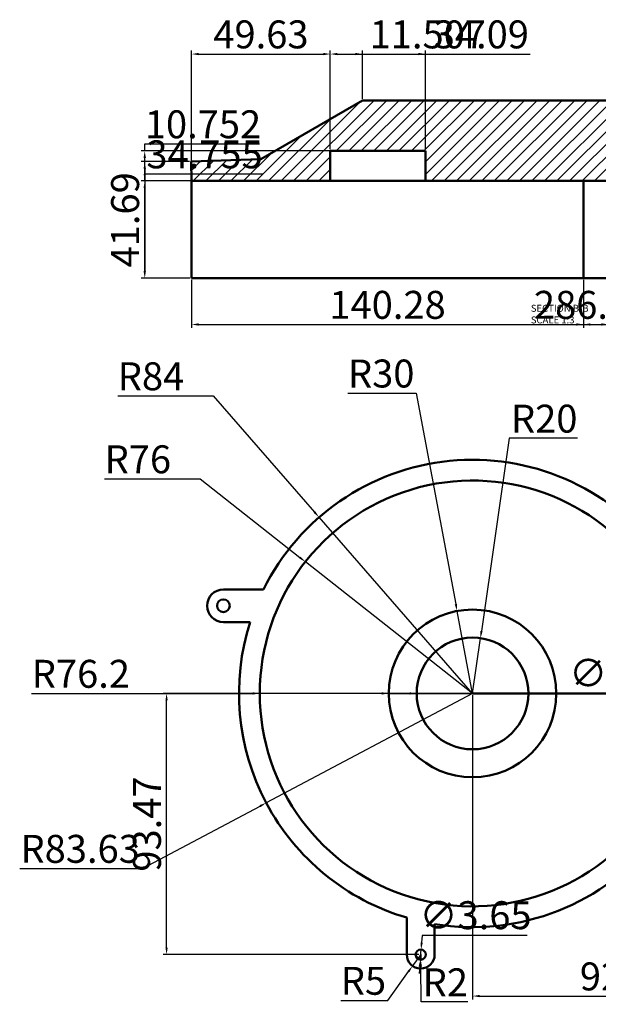
# Model space of a CAD drawing. Units: millimetres. Extents: x 828 to 2987, y 979 to 1807.
# Tile 1 of 6: x 851 to 1058, y 1108 to 1460. Entities that reach past the tile are written whole.
import ezdxf

# ---------------------------------------------------------------- set-up
doc = ezdxf.new("R2010")
doc.units = ezdxf.units.MM
for name, color, linetype, lineweight in [('M-DIMS', 2, 'Continuous', 25), ('M-HATC', 8, 'Continuous', 18), ('M-OUTL', 7, 'Continuous', 50), ('M-TEXT', 3, 'Continuous', 25)]:
    doc.layers.add(name, color=color, linetype=linetype, lineweight=lineweight)
doc.styles.get("Standard").update_dxf_attribs({"font": 'arial.ttf'})
doc.dimstyles.new('ISO-25', dxfattribs={"dimtxt": 10, "dimasz": 2.5, "dimexe": 1.25, "dimexo": 0.625, "dimtad": 1, "dimtoh": 1, "dimdec": 0, "dimtxsty": 'Standard', "dimcen": 2.5, "dimadec": 0, "dimazin": 0, "dimtfac": 1, "dimtdec": 0, "dimtmove": 0, "dimatfit": 3, "dimfxl": 1, "dimarcsym": 0})

# ---------------------------------------------------------------- blocks, each defined once
blk = doc.blocks.new('*D17')
at = {"layer": 'Defpoints', "color": 0, "transparency": 16777216}
for p in [(1013.21, 1219.26), (1105.21, 1219.26), (1105.21, 1110.96)]:
    blk.add_point(p, dxfattribs=at)
at = {"layer": 'M-DIMS', "color": 0, "lineweight": -2, "transparency": 16777216}
for p, q in [((1013.21, 1218.63), (1013.21, 1109.71)), ((1105.21, 1218.63), (1105.21, 1109.71)), ((1015.71, 1110.96), (1102.71, 1110.96))]:
    blk.add_line(p, q, dxfattribs=at)
at = {"layer": 'M-DIMS', "color": 0, "transparency": 16777216}
for points in [[(1015.71, 1111.37), (1015.71, 1110.54), (1013.21, 1110.96)], [(1102.71, 1111.37), (1102.71, 1110.54), (1105.21, 1110.96)]]:
    blk.add_solid(points, dxfattribs=at)
at = {"layer": 'M-DIMS', "color": 0, "transparency": 16777216, "insert": (1059.21, 1116.69), "char_height": 10, "attachment_point": 5}
blk.add_mtext('92', dxfattribs=at)
blk = doc.blocks.new('*D18')
at = {"layer": 'Defpoints', "color": 0, "transparency": 16777216}
for p in [(958.25, 1282.29), (1013.21, 1219.26)]:
    blk.add_point(p, dxfattribs=at)
at = {"layer": 'M-DIMS', "color": 0, "lineweight": -2, "transparency": 16777216}
for p, q in [((886.14, 1325.74), (920.35, 1325.74)), ((920.35, 1325.74), (956.61, 1284.17)), ((1013.21, 1219.26), (958.25, 1282.29))]:
    blk.add_line(p, q, dxfattribs=at)
at = {"layer": 'M-DIMS', "color": 0, "transparency": 16777216}
blk.add_solid([(956.92, 1284.44), (956.29, 1283.9), (958.25, 1282.29)], dxfattribs=at)
at = {"layer": 'M-DIMS', "color": 0, "transparency": 16777216, "insert": (898.07, 1331.47), "char_height": 10, "attachment_point": 5}
blk.add_mtext('R84', dxfattribs=at)
blk = doc.blocks.new('*D19')
at = {"layer": 'Defpoints', "color": 0, "transparency": 16777216}
for p in [(953.34, 1266.38), (1013.21, 1219.26)]:
    blk.add_point(p, dxfattribs=at)
at = {"layer": 'M-DIMS', "color": 0, "lineweight": -2, "transparency": 16777216}
for p, q in [((881.42, 1296.03), (915.66, 1296.03)), ((915.66, 1296.03), (951.37, 1267.92)), ((1013.21, 1219.26), (953.34, 1266.38))]:
    blk.add_line(p, q, dxfattribs=at)
at = {"layer": 'M-DIMS', "color": 0, "transparency": 16777216}
blk.add_solid([(951.63, 1268.25), (951.11, 1267.59), (953.34, 1266.38)], dxfattribs=at)
at = {"layer": 'M-DIMS', "color": 0, "transparency": 16777216, "insert": (893.36, 1301.76), "char_height": 10, "attachment_point": 5}
blk.add_mtext('R76', dxfattribs=at)
blk = doc.blocks.new('*D25')
at = {"layer": 'Defpoints', "color": 0, "transparency": 16777216}
for p in [(994.65, 1125.79), (991.73, 1121.73)]:
    blk.add_point(p, dxfattribs=at)
at = {"layer": 'M-DIMS', "color": 0, "lineweight": -2, "transparency": 16777216}
for p, q in [((994.65, 1125.79), (991.73, 1121.73)), ((982.88, 1109.41), (990.27, 1119.7)), ((966.05, 1109.41), (982.88, 1109.41))]:
    blk.add_line(p, q, dxfattribs=at)
at = {"layer": 'M-DIMS', "color": 0, "transparency": 16777216}
blk.add_solid([(989.93, 1119.94), (990.61, 1119.45), (991.73, 1121.73)], dxfattribs=at)
at = {"layer": 'M-DIMS', "color": 0, "transparency": 16777216, "insert": (974.15, 1115.12), "char_height": 10, "attachment_point": 5}
blk.add_mtext('R5', dxfattribs=at)
blk = doc.blocks.new('*D26')
at = {"layer": 'Defpoints', "color": 0, "transparency": 16777216}
for p in [(994.65, 1125.79), (994.67, 1123.96)]:
    blk.add_point(p, dxfattribs=at)
at = {"layer": 'M-DIMS', "color": 0, "lineweight": -2, "transparency": 16777216}
for p, q in [((994.65, 1125.79), (994.67, 1123.96)), ((994.83, 1108.92), (994.69, 1121.46)), ((1011.47, 1108.92), (994.83, 1108.92))]:
    blk.add_line(p, q, dxfattribs=at)
at = {"layer": 'M-DIMS', "color": 0, "transparency": 16777216}
blk.add_solid([(995.11, 1121.47), (994.28, 1121.46), (994.67, 1123.96)], dxfattribs=at)
at = {"layer": 'M-DIMS', "color": 0, "transparency": 16777216, "insert": (1003.46, 1114.57), "char_height": 10, "attachment_point": 5}
blk.add_mtext('R2', dxfattribs=at)
blk = doc.blocks.new('*D27')
at = {"layer": 'Defpoints', "color": 0, "transparency": 16777216}
for p in [(1007.69, 1248.75), (1013.21, 1219.26)]:
    blk.add_point(p, dxfattribs=at)
at = {"layer": 'M-DIMS', "color": 0, "lineweight": -2, "transparency": 16777216}
for p, q in [((968.58, 1326.71), (993.07, 1326.71)), ((993.07, 1326.71), (1007.23, 1251.2)), ((1013.21, 1219.26), (1007.69, 1248.75))]:
    blk.add_line(p, q, dxfattribs=at)
at = {"layer": 'M-DIMS', "color": 0, "transparency": 16777216}
blk.add_solid([(1007.64, 1251.28), (1006.82, 1251.13), (1007.69, 1248.75)], dxfattribs=at)
at = {"layer": 'M-DIMS', "color": 0, "transparency": 16777216, "insert": (980.51, 1332.45), "char_height": 10, "attachment_point": 5}
blk.add_mtext('R30', dxfattribs=at)
blk = doc.blocks.new('*D28')
at = {"layer": 'Defpoints', "color": 0, "transparency": 16777216}
for p in [(1016.06, 1239.06), (1013.21, 1219.26)]:
    blk.add_point(p, dxfattribs=at)
at = {"layer": 'M-DIMS', "color": 0, "lineweight": -2, "transparency": 16777216}
for p, q in [((1026.32, 1310.58), (1016.41, 1241.53)), ((1050.81, 1310.58), (1026.32, 1310.58)), ((1013.21, 1219.26), (1016.06, 1239.06))]:
    blk.add_line(p, q, dxfattribs=at)
at = {"layer": 'M-DIMS', "color": 0, "transparency": 16777216}
blk.add_solid([(1016, 1241.59), (1016.82, 1241.47), (1016.06, 1239.06)], dxfattribs=at)
at = {"layer": 'M-DIMS', "color": 0, "transparency": 16777216, "insert": (1038.88, 1316.31), "char_height": 10, "attachment_point": 5}
blk.add_mtext('R20', dxfattribs=at)
blk = doc.blocks.new('*D77')
at = {"layer": 'Defpoints', "color": 0, "transparency": 16777216}
for p in [(903.65, 1219.26), (1013.21, 1219.26), (994.65, 1125.79)]:
    blk.add_point(p, dxfattribs=at)
at = {"layer": 'M-DIMS', "color": 0, "lineweight": -2, "transparency": 16777216}
for p, q in [((1012.59, 1219.26), (902.4, 1219.26)), ((903.65, 1128.29), (903.65, 1216.76)), ((994.02, 1125.79), (902.4, 1125.79))]:
    blk.add_line(p, q, dxfattribs=at)
at = {"layer": 'M-DIMS', "color": 0, "transparency": 16777216}
for points in [[(903.24, 1216.76), (904.07, 1216.76), (903.65, 1219.26)], [(903.24, 1128.29), (904.07, 1128.29), (903.65, 1125.79)]]:
    blk.add_solid(points, dxfattribs=at)
at = {"layer": 'M-DIMS', "color": 0, "transparency": 16777216, "insert": (897.92, 1172.52), "char_height": 10, "attachment_point": 5, "rotation": 90}
blk.add_mtext('93.47', dxfattribs=at)
blk = doc.blocks.new('*D80')
at = {"layer": 'Defpoints', "color": 0, "transparency": 16777216}
for p in [(912.63, 1367.9), (1199.4, 1367.9), (1199.4, 1351.3)]:
    blk.add_point(p, dxfattribs=at)
at = {"layer": 'M-DIMS', "color": 0, "lineweight": -2, "transparency": 16777216}
for p, q in [((912.63, 1367.28), (912.63, 1350.05)), ((1199.4, 1367.28), (1199.4, 1350.05)), ((915.13, 1351.3), (1196.9, 1351.3))]:
    blk.add_line(p, q, dxfattribs=at)
at = {"layer": 'M-DIMS', "color": 0, "transparency": 16777216}
for points in [[(915.13, 1351.72), (915.13, 1350.88), (912.63, 1351.3)], [(1196.9, 1351.72), (1196.9, 1350.88), (1199.4, 1351.3)]]:
    blk.add_solid(points, dxfattribs=at)
at = {"layer": 'M-DIMS', "color": 0, "transparency": 16777216, "insert": (1056.02, 1357.03), "char_height": 10, "attachment_point": 5}
blk.add_mtext('286.76', dxfattribs=at)
blk = doc.blocks.new('*D82')
at = {"layer": 'Defpoints', "color": 0, "transparency": 16777216}
for p in [(895.83, 1402.66), (912.63, 1402.66), (912.63, 1367.9)]:
    blk.add_point(p, dxfattribs=at)
at = {"layer": 'M-DIMS', "color": 0, "lineweight": -2, "transparency": 16777216}
for p, q in [((912.01, 1402.66), (894.58, 1402.66)), ((895.83, 1402.66), (895.83, 1405.16)), ((895.83, 1405.16), (938.04, 1405.16)), ((895.83, 1370.4), (895.83, 1400.16)), ((912.01, 1367.9), (894.58, 1367.9))]:
    blk.add_line(p, q, dxfattribs=at)
at = {"layer": 'M-DIMS', "color": 0, "transparency": 16777216}
for points in [[(895.42, 1400.16), (896.25, 1400.16), (895.83, 1402.66)], [(895.42, 1370.4), (896.25, 1370.4), (895.83, 1367.9)]]:
    blk.add_solid(points, dxfattribs=at)
at = {"layer": 'M-DIMS', "color": 0, "transparency": 16777216, "insert": (917.25, 1410.89), "char_height": 10, "attachment_point": 5}
blk.add_mtext('34.755', dxfattribs=at)
blk = doc.blocks.new('*D83')
at = {"layer": 'Defpoints', "color": 0, "transparency": 16777216}
for p in [(912.43, 1409.59), (895.83, 1367.9), (912.63, 1367.9)]:
    blk.add_point(p, dxfattribs=at)
at = {"layer": 'M-DIMS', "color": 0, "lineweight": -2, "transparency": 16777216}
for p, q in [((911.81, 1409.59), (894.58, 1409.59)), ((895.83, 1407.09), (895.83, 1370.4)), ((912.01, 1367.9), (894.58, 1367.9))]:
    blk.add_line(p, q, dxfattribs=at)
at = {"layer": 'M-DIMS', "color": 0, "transparency": 16777216}
for points in [[(895.42, 1407.09), (896.25, 1407.09), (895.83, 1409.59)], [(895.42, 1370.4), (896.25, 1370.4), (895.83, 1367.9)]]:
    blk.add_solid(points, dxfattribs=at)
at = {"layer": 'M-DIMS', "color": 0, "transparency": 16777216, "insert": (890.1, 1388.75), "char_height": 10, "attachment_point": 5, "rotation": 90}
blk.add_mtext('41.69', dxfattribs=at)
blk = doc.blocks.new('*D84')
at = {"layer": 'Defpoints', "color": 0, "transparency": 16777216}
for p in [(973.77, 1448.08), (973.77, 1431.48), (962.27, 1413.41)]:
    blk.add_point(p, dxfattribs=at)
at = {"layer": 'M-DIMS', "color": 0, "lineweight": -2, "transparency": 16777216}
for p, q in [((962.27, 1414.03), (962.27, 1449.33)), ((973.77, 1432.11), (973.77, 1449.33)), ((964.77, 1448.08), (971.27, 1448.08)), ((973.77, 1448.08), (1018.1, 1448.08))]:
    blk.add_line(p, q, dxfattribs=at)
at = {"layer": 'M-DIMS', "color": 0, "transparency": 16777216}
for points in [[(964.77, 1448.5), (964.77, 1447.67), (962.27, 1448.08)], [(971.27, 1448.5), (971.27, 1447.67), (973.77, 1448.08)]]:
    blk.add_solid(points, dxfattribs=at)
at = {"layer": 'M-DIMS', "color": 0, "transparency": 16777216, "insert": (997.19, 1453.81), "char_height": 10, "attachment_point": 5}
blk.add_mtext('11.507', dxfattribs=at)
blk = doc.blocks.new('*D85')
at = {"layer": 'Defpoints', "color": 0, "transparency": 16777216}
for p in [(962.27, 1448.08), (962.27, 1413.41), (912.63, 1402.66)]:
    blk.add_point(p, dxfattribs=at)
at = {"layer": 'M-DIMS', "color": 0, "lineweight": -2, "transparency": 16777216}
for p, q in [((912.63, 1403.28), (912.63, 1449.33)), ((962.27, 1414.03), (962.27, 1449.33)), ((915.13, 1448.08), (959.77, 1448.08))]:
    blk.add_line(p, q, dxfattribs=at)
at = {"layer": 'M-DIMS', "color": 0, "transparency": 16777216}
for points in [[(915.13, 1448.5), (915.13, 1447.67), (912.63, 1448.08)], [(959.77, 1448.5), (959.77, 1447.67), (962.27, 1448.08)]]:
    blk.add_solid(points, dxfattribs=at)
at = {"layer": 'M-DIMS', "color": 0, "transparency": 16777216, "insert": (937.45, 1453.82), "char_height": 10, "attachment_point": 5}
blk.add_mtext('49.63', dxfattribs=at)
blk = doc.blocks.new('*D86')
at = {"layer": 'Defpoints', "color": 0, "transparency": 16777216}
for p in [(996.36, 1448.08), (962.27, 1413.41), (996.36, 1413.41)]:
    blk.add_point(p, dxfattribs=at)
at = {"layer": 'M-DIMS', "color": 0, "lineweight": -2, "transparency": 16777216}
for p, q in [((962.27, 1414.03), (962.27, 1449.33)), ((996.36, 1414.03), (996.36, 1449.33)), ((964.77, 1448.08), (993.86, 1448.08)), ((996.36, 1448.08), (1033.87, 1448.08))]:
    blk.add_line(p, q, dxfattribs=at)
at = {"layer": 'M-DIMS', "color": 0, "transparency": 16777216}
for points in [[(964.77, 1448.5), (964.77, 1447.67), (962.27, 1448.08)], [(993.86, 1448.5), (993.86, 1447.67), (996.36, 1448.08)]]:
    blk.add_solid(points, dxfattribs=at)
at = {"layer": 'M-DIMS', "color": 0, "transparency": 16777216, "insert": (1016.36, 1453.82), "char_height": 10, "attachment_point": 5}
blk.add_mtext('34.09', dxfattribs=at)
blk = doc.blocks.new('*D87')
at = {"layer": 'Defpoints', "color": 0, "transparency": 16777216}
for p in [(895.83, 1413.41), (996.36, 1413.41), (996.36, 1402.66)]:
    blk.add_point(p, dxfattribs=at)
at = {"layer": 'M-DIMS', "color": 0, "lineweight": -2, "transparency": 16777216}
for p, q in [((995.73, 1413.41), (894.58, 1413.41)), ((895.83, 1413.41), (895.83, 1415.91)), ((895.83, 1415.91), (936.93, 1415.91)), ((895.83, 1405.16), (895.83, 1410.91)), ((995.73, 1402.66), (894.58, 1402.66))]:
    blk.add_line(p, q, dxfattribs=at)
at = {"layer": 'M-DIMS', "color": 0, "transparency": 16777216}
for points in [[(895.42, 1410.91), (896.25, 1410.91), (895.83, 1413.41)], [(895.42, 1405.16), (896.25, 1405.16), (895.83, 1402.66)]]:
    blk.add_solid(points, dxfattribs=at)
at = {"layer": 'M-DIMS', "color": 0, "transparency": 16777216, "insert": (916.69, 1421.64), "char_height": 10, "attachment_point": 5}
blk.add_mtext('10.752', dxfattribs=at)
blk = doc.blocks.new('*D91')
at = {"layer": 'Defpoints', "color": 0, "transparency": 16777216}
for p in [(912.63, 1367.9), (1052.92, 1367.9), (1052.92, 1351.3)]:
    blk.add_point(p, dxfattribs=at)
at = {"layer": 'M-DIMS', "color": 0, "lineweight": -2, "transparency": 16777216}
for p, q in [((912.63, 1367.28), (912.63, 1350.05)), ((1052.92, 1367.28), (1052.92, 1350.05)), ((915.13, 1351.3), (1050.42, 1351.3))]:
    blk.add_line(p, q, dxfattribs=at)
at = {"layer": 'M-DIMS', "color": 0, "transparency": 16777216}
for points in [[(915.13, 1351.72), (915.13, 1350.88), (912.63, 1351.3)], [(1050.42, 1351.72), (1050.42, 1350.88), (1052.92, 1351.3)]]:
    blk.add_solid(points, dxfattribs=at)
at = {"layer": 'M-DIMS', "color": 0, "transparency": 16777216, "insert": (982.78, 1357.03), "char_height": 10, "attachment_point": 5}
blk.add_mtext('140.28', dxfattribs=at)
blk = doc.blocks.new('*D92')
at = {"layer": 'Defpoints', "color": 0, "transparency": 16777216}
for p in [(1052.92, 1367.9), (1061.89, 1367.9), (1061.89, 1351.3)]:
    blk.add_point(p, dxfattribs=at)
at = {"layer": 'M-DIMS', "color": 0, "lineweight": -2, "transparency": 16777216}
for p, q in [((1052.92, 1367.28), (1052.92, 1350.05)), ((1061.89, 1367.28), (1061.89, 1350.05)), ((1055.42, 1351.3), (1059.39, 1351.3)), ((1061.89, 1351.3), (1091.63, 1351.3))]:
    blk.add_line(p, q, dxfattribs=at)
at = {"layer": 'M-DIMS', "color": 0, "transparency": 16777216}
for points in [[(1055.42, 1351.72), (1055.42, 1350.88), (1052.92, 1351.3)], [(1059.39, 1351.72), (1059.39, 1350.88), (1061.89, 1351.3)]]:
    blk.add_solid(points, dxfattribs=at)
at = {"layer": 'M-DIMS', "color": 0, "transparency": 16777216, "insert": (1078.01, 1357.03), "char_height": 10, "attachment_point": 5}
blk.add_mtext('8.97', dxfattribs=at)
blk = doc.blocks.new('*D124')
at = {"layer": 'Defpoints', "color": 0, "transparency": 16777216}
for p in [(1013.21, 1219.26), (939.32, 1180.1)]:
    blk.add_point(p, dxfattribs=at)
at = {"layer": 'M-DIMS', "color": 0, "lineweight": -2, "transparency": 16777216}
for p, q in [((1013.21, 1219.26), (939.32, 1180.1)), ((894.99, 1156.6), (937.12, 1178.93)), ((851.05, 1156.6), (894.99, 1156.6))]:
    blk.add_line(p, q, dxfattribs=at)
at = {"layer": 'M-DIMS', "color": 0, "transparency": 16777216}
blk.add_solid([(936.92, 1179.3), (937.31, 1178.56), (939.32, 1180.1)], dxfattribs=at)
at = {"layer": 'M-DIMS', "color": 0, "transparency": 16777216, "insert": (872.71, 1162.34), "char_height": 10, "attachment_point": 5}
blk.add_mtext('R83.63', dxfattribs=at)
blk = doc.blocks.new('*D125')
at = {"layer": 'Defpoints', "color": 0, "transparency": 16777216}
for p in [(937.02, 1219.26), (1013.21, 1219.26)]:
    blk.add_point(p, dxfattribs=at)
at = {"layer": 'M-DIMS', "color": 0, "lineweight": -2, "transparency": 16777216}
for p, q in [((855.24, 1219.26), (891.31, 1219.26)), ((891.31, 1219.26), (934.52, 1219.26)), ((1013.21, 1219.26), (937.02, 1219.26))]:
    blk.add_line(p, q, dxfattribs=at)
at = {"layer": 'M-DIMS', "color": 0, "transparency": 16777216}
blk.add_solid([(934.52, 1219.68), (934.52, 1218.84), (937.02, 1219.26)], dxfattribs=at)
at = {"layer": 'M-DIMS', "color": 0, "transparency": 16777216, "insert": (872.96, 1224.99), "char_height": 10, "attachment_point": 5}
blk.add_mtext('R76.2', dxfattribs=at)
blk = doc.blocks.new('*D126')
at = {"layer": 'Defpoints', "color": 0, "transparency": 16777216}
for p in [(983.21, 1219.26), (1043.21, 1219.26)]:
    blk.add_point(p, dxfattribs=at)
at = {"layer": 'M-DIMS', "color": 0, "lineweight": -2, "transparency": 16777216}
for p, q in [((980.71, 1219.26), (978.21, 1219.26)), ((983.21, 1219.26), (1043.21, 1219.26)), ((1061.21, 1219.26), (1045.71, 1219.26)), ((1087.01, 1219.26), (1061.21, 1219.26))]:
    blk.add_line(p, q, dxfattribs=at)
at = {"layer": 'M-DIMS', "color": 0, "transparency": 16777216}
for points in [[(980.71, 1219.68), (980.71, 1218.84), (983.21, 1219.26)], [(1045.71, 1219.68), (1045.71, 1218.84), (1043.21, 1219.26)]]:
    blk.add_solid(points, dxfattribs=at)
at = {"layer": 'M-DIMS', "color": 0, "transparency": 16777216, "insert": (1074.43, 1225.27), "char_height": 10, "attachment_point": 5}
blk.add_mtext('∅60', dxfattribs=at)
blk = doc.blocks.new('*D127')
at = {"layer": 'Defpoints', "color": 0, "transparency": 16777216}
for p in [(993.21, 1219.26), (1033.21, 1219.26)]:
    blk.add_point(p, dxfattribs=at)
at = {"layer": 'M-DIMS', "color": 0, "lineweight": -2, "transparency": 16777216}
for p, q in [((990.71, 1219.26), (988.21, 1219.26)), ((993.21, 1219.26), (1033.21, 1219.26)), ((1048.99, 1219.26), (1035.71, 1219.26)), ((1074.78, 1219.26), (1048.99, 1219.26))]:
    blk.add_line(p, q, dxfattribs=at)
at = {"layer": 'M-DIMS', "color": 0, "transparency": 16777216}
for points in [[(990.71, 1219.68), (990.71, 1218.84), (993.21, 1219.26)], [(1035.71, 1219.68), (1035.71, 1218.84), (1033.21, 1219.26)]]:
    blk.add_solid(points, dxfattribs=at)
at = {"layer": 'M-DIMS', "color": 0, "transparency": 16777216, "insert": (1062.2, 1225.27), "char_height": 10, "attachment_point": 5}
blk.add_mtext('∅40', dxfattribs=at)
blk = doc.blocks.new('*D132')
at = {"layer": 'Defpoints', "color": 0, "transparency": 16777216}
for p in [(994.79, 1127.61), (994.51, 1123.97)]:
    blk.add_point(p, dxfattribs=at)
at = {"layer": 'M-DIMS', "color": 0, "lineweight": -2, "transparency": 16777216}
for p, q in [((995.19, 1132.59), (994.99, 1130.1)), ((1032.74, 1132.59), (995.19, 1132.59)), ((994.51, 1123.97), (994.79, 1127.61)), ((994.31, 1121.48), (994.11, 1118.98))]:
    blk.add_line(p, q, dxfattribs=at)
at = {"layer": 'M-DIMS', "color": 0, "transparency": 16777216}
for points in [[(994.57, 1130.13), (995.4, 1130.07), (994.79, 1127.61)], [(993.89, 1121.51), (994.72, 1121.44), (994.51, 1123.97)]]:
    blk.add_solid(points, dxfattribs=at)
at = {"layer": 'M-DIMS', "color": 0, "transparency": 16777216, "insert": (1014.28, 1138.6), "char_height": 10, "attachment_point": 5}
blk.add_mtext('∅3.65', dxfattribs=at)

msp = doc.modelspace()

# ---------------------------------------------------------------- hatches: boundary and pattern name
at = {"layer": 'M-HATC'}
h = msp.add_hatch(dxfattribs=at)
h.set_pattern_fill('ANSI31', color=256)
h.paths.add_polyline_path([(962.2684, 1413.4084), (996.3583, 1413.4084), (996.3583, 1402.6561), (1084.8819, 1402.6561), (1084.8819, 1414.7818), (1117.3222, 1414.7818), (1117.3222, 1402.6561), (1194.3976, 1402.6561), (1194.3976, 1367.9009), (1199.3976, 1367.9009), (1199.3976, 1423.4818, -0.41421356), (1191.3976, 1431.4818), (1171.0768, 1431.4818), (1161.8287, 1415.4895, -0.59566696), (1156.5548, 1415.6369), (1148.5383, 1431.4818), (973.775, 1431.4818), (937.4085, 1410.469), (912.4339, 1409.5934), (912.6342, 1402.6561), (962.2684, 1402.6561)])

# ---------------------------------------------------------------- linework, layer by layer
at = {"layer": 'M-OUTL'}
for p, q in [((973.775, 1431.4818), (937.4085, 1410.469)), ((1191.3976, 1431.4818), (973.775, 1431.4818)), ((962.2684, 1402.6561), (962.2684, 1413.4084)), ((962.2684, 1413.4084), (996.3583, 1413.4084)), ((996.3583, 1413.4084), (996.3583, 1402.6561)), ((937.4085, 1410.469), (912.4339, 1409.5934)), ((912.4339, 1409.5934), (912.6342, 1402.6561)), ((1194.3976, 1402.6561), (912.6342, 1402.6561)), ((912.6342, 1367.9009), (912.6342, 1402.6561)), ((1052.9164, 1367.9009), (1052.9164, 1402.6561)), ((912.6342, 1367.9009), (1194.3976, 1367.9009)), ((923.9922, 1256.4847), (938.3309, 1256.4847)), ((923.9922, 1244.804), (933.5857, 1244.804)), ((1013.2149, 1219.2594), (1105.2149, 1219.2594)), ((989.6492, 1125.7871), (989.6492, 1139.0223)), ((999.6492, 1125.7871), (999.6492, 1136.7409))]:
    msp.add_line(p, q, dxfattribs=at)
for centre, radius in [((923.9922, 1250.6444), 2.2667), ((1013.2149, 1219.2594), 30), ((1013.2149, 1219.2594), 20), ((994.6492, 1125.7871), 1.8253)]:
    msp.add_circle(centre, radius, dxfattribs=at)
for centre, radius, start, end in [((1013.2149, 1219.2594), 83.6262, 37.706236, 153.567782), ((1013.2149, 1219.2594), 76.1927, 33.749512, 326.250488), ((923.9922, 1250.6444), 5.8403, 90, 270), ((1013.2149, 1219.2594), 83.6262, 162.214047, 253.632492), ((1013.2149, 1219.2594), 83.6262, 260.664363, 322.293764), ((994.6492, 1125.7871), 5, 180, 0)]:
    msp.add_arc(centre, radius, start, end, dxfattribs=at)

# ---------------------------------------------------------------- texts
at = {"layer": 'M-TEXT', "insert": (1034.0859, 1358.3458), "char_height": 2.5, "attachment_point": 1}
msp.add_mtext_dynamic_manual_height_columns('SECTION B-B\\PSCALE 1:3', width=102.622047, gutter_width=12.5, heights=[0], dxfattribs=at)

# ---------------------------------------------------------------- dimensions: what is measured, and where the dimension line sits
at = {"layer": 'M-DIMS'}
for base, p1, p2, override, picture, middle in [((962.2684, 1448.0818), (912.6342, 1402.6561), (962.2684, 1413.4084), {"dimdec": 2, "dimlfac": 1, "dimrnd": 0, "dimzin": 0, "dimdsep": 46, "dimlunit": 2}, '*D85', (937.4513, 1453.816)), ((996.3583, 1448.0818), (962.2684, 1413.4084), (996.3583, 1413.4084), {"dimdec": 2, "dimlfac": 1, "dimrnd": 0, "dimzin": 0, "dimdsep": 46, "dimlunit": 2}, '*D86', (1016.3625, 1453.816)), ((973.775, 1448.0818), (962.2684, 1413.4084), (973.775, 1431.4818), {"dimdec": 3, "dimlfac": 1, "dimrnd": 0, "dimzin": 0, "dimdsep": 46, "dimlunit": 2}, '*D84', (997.1865, 1453.8126)), ((1199.3976, 1351.3009), (912.6342, 1367.9009), (1199.3976, 1367.9009), {"dimdec": 2, "dimlfac": 1, "dimrnd": 0, "dimzin": 0, "dimdsep": 46, "dimlunit": 2}, '*D80', (1056.0159, 1357.0316)), ((1052.9164, 1351.3009), (912.6342, 1367.9009), (1052.9164, 1367.9009), {"dimdec": 2, "dimlfac": 1, "dimrnd": 0, "dimzin": 0, "dimdsep": 46, "dimlunit": 2}, '*D91', (982.7753, 1357.0316)), ((1061.8863, 1351.3009), (1052.9164, 1367.9009), (1061.8863, 1367.9009), {"dimdec": 2, "dimlfac": 1, "dimrnd": 0, "dimzin": 0, "dimdsep": 46, "dimlunit": 2}, '*D92', (1078.0058, 1357.0316)), ((1105.2149, 1110.9564), (1013.2149, 1219.2594), (1105.2149, 1219.2594), {"dimclrd": 0, "dimclre": 0, "dimclrt": 0}, '*D17', (1059.2149, 1116.6871))]:
    dim = msp.add_linear_dim(base=base, p1=p1, p2=p2, dimstyle='ISO-25', override=override, dxfattribs=at)
    dim.commit()
    dim.dimension.update_dxf_attribs({"geometry": picture, "text_midpoint": middle})
for base, p1, p2, override, picture, middle in [((895.8339, 1413.4084), (996.3583, 1402.6561), (996.3583, 1413.4084), {"dimdec": 3, "dimlfac": 1, "dimrnd": 0, "dimzin": 0, "dimdsep": 46, "dimlunit": 2}, '*D87', (916.6942, 1421.6391)), ((895.8339, 1402.6561), (912.6342, 1367.9009), (912.6342, 1402.6561), {"dimdec": 3, "dimlfac": 1, "dimrnd": 0, "dimzin": 0, "dimdsep": 46, "dimlunit": 2}, '*D82', (917.2501, 1410.8903)), ((895.8339, 1367.9009), (912.4339, 1409.5934), (912.6342, 1367.9009), {"dimdec": 2, "dimlfac": 1, "dimrnd": 0, "dimzin": 0, "dimdsep": 46, "dimlunit": 2}, '*D83', (890.1031, 1388.7472)), ((903.6518, 1219.2594), (994.6492, 1125.7871), (1013.2149, 1219.2594), {"dimdec": 2, "dimlfac": 1, "dimrnd": 0, "dimzin": 0, "dimdsep": 46, "dimlunit": 2}, '*D77', (897.9177, 1172.5233))]:
    dim = msp.add_linear_dim(base=base, p1=p1, p2=p2, angle=90, dimstyle='ISO-25', override=override, dxfattribs=at)
    dim.commit()
    dim.dimension.update_dxf_attribs({"geometry": picture, "text_midpoint": middle})
for mpoint, override, picture, middle in [((958.2508, 1282.2855), {"dimclrd": 0, "dimclre": 0, "dimclrt": 0}, '*D18', (898.0711, 1325.7412)), ((1007.687, 1248.7457), {"dimclrd": 0, "dimclre": 0, "dimclrt": 0}, '*D27', (980.5148, 1326.7125)), ((1016.0563, 1239.0566), {"dimclrd": 0, "dimclre": 0, "dimclrt": 0}, '*D28', (1038.8768, 1310.5778)), ((953.3372, 1266.3763), {"dimclrd": 0, "dimclre": 0, "dimclrt": 0}, '*D19', (893.3649, 1296.0258)), ((937.0221, 1219.259), {"dimdec": 1, "dimlfac": 1, "dimrnd": 0, "dimzin": 0, "dimdsep": 46, "dimlunit": 2}, '*D125', (891.3065, 1219.2587)), ((939.325, 1180.098), {"dimdec": 2, "dimlfac": 1, "dimrnd": 0, "dimzin": 0, "dimdsep": 46, "dimlunit": 2}, '*D124', (872.7085, 1156.6011))]:
    dim = msp.add_radius_dim(center=(1013.2149, 1219.2594), mpoint=mpoint, dimstyle='ISO-25', override=override, dxfattribs=at)
    dim.commit()
    dim.dimension.update_dxf_attribs({"geometry": picture, "text_midpoint": middle, "dimtype": 164})
for p1, p2, override, picture, middle in [((983.2149, 1219.2599), (1043.2149, 1219.259), {"dimdec": 0, "dimlfac": 1, "dimrnd": 0, "dimzin": 0, "dimdsep": 46, "dimlunit": 2}, '*D126', (1061.2149, 1219.2587)), ((994.5058, 1123.9674), (994.7927, 1127.6068), {"dimdec": 2, "dimlfac": 1, "dimrnd": 0, "dimzin": 0, "dimdsep": 46, "dimlunit": 2}, '*D132', (1014.2757, 1132.5913))]:
    dim = msp.add_diameter_dim_2p(p1=p1, p2=p2, dimstyle='ISO-25', override=override, dxfattribs=at)
    dim.commit()
    dim.dimension.update_dxf_attribs({"geometry": picture, "text_midpoint": middle, "dimtype": 163})
dim = msp.add_diameter_dim_2p(p1=(993.2149, 1219.2599), p2=(1033.2149, 1219.259), dimstyle='ISO-25', override={"dimdec": 0, "dimlfac": 1, "dimrnd": 0, "dimzin": 0, "dimdsep": 46, "dimlunit": 2}, dxfattribs=at)
dim.commit()
dim.dimension.update_dxf_attribs({"geometry": '*D127', "text_midpoint": (1048.9857, 1219.2587)})
for mpoint, picture, middle in [((991.7312, 1121.7269), '*D25', (974.1523, 1115.1182)), ((994.6684, 1123.9619), '*D26', (1003.4627, 1114.5673))]:
    dim = msp.add_radius_dim(center=(994.6492, 1125.7871), mpoint=mpoint, dimstyle='ISO-25', override={"dimclrd": 0, "dimclre": 0, "dimclrt": 0}, dxfattribs=at)
    dim.commit()
    dim.dimension.update_dxf_attribs({"geometry": picture, "text_midpoint": middle})

doc.saveas('drawing.dxf')
